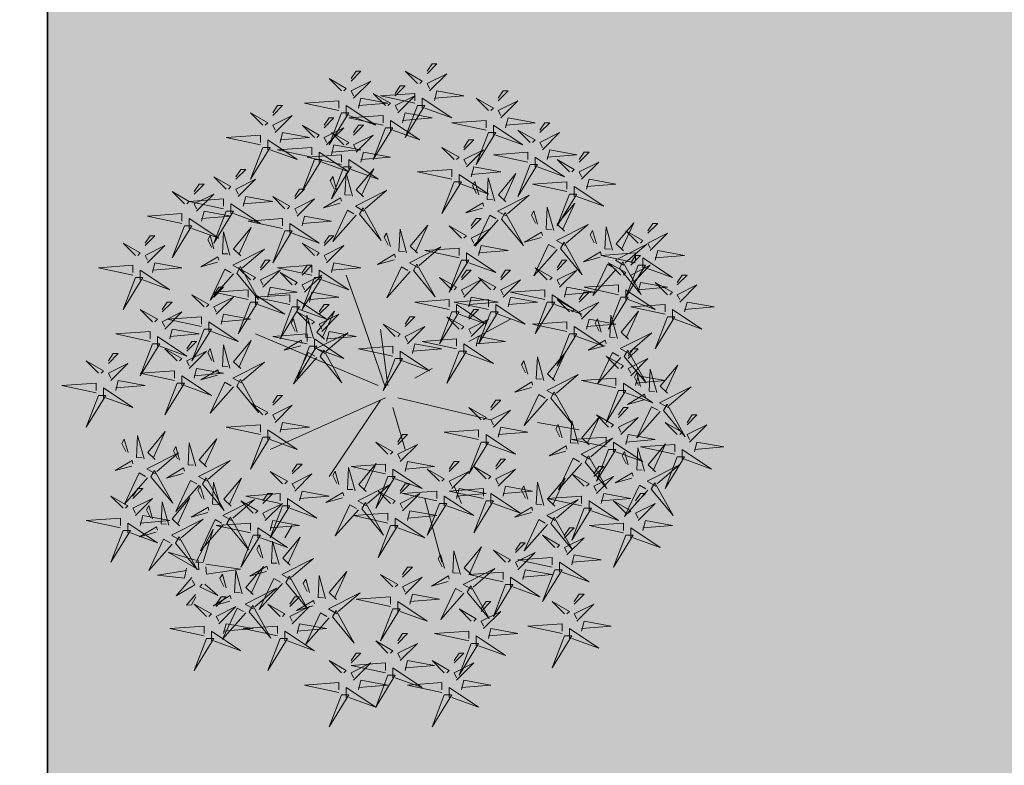
# Model space of a CAD drawing. Units: inches. Extents: x 1704 to 6393, y -157 to 1172.
# Tile 64 of 122: x 1897 to 1937, y 920 to 950. Entities that reach past the tile are written whole.
import ezdxf

# ---------------------------------------------------------------- set-up
doc = ezdxf.new("R2010")
doc.units = ezdxf.units.IN
doc.header["$MEASUREMENT"] = 0
for name, color, linetype, lineweight in [('A-ANNO-DIMS', 7, 'Continuous', 13), ('C-PROP', 7, 'Continuous', 35), ('L-shrub', 74, 'Continuous', 18)]:
    doc.layers.add(name, color=color, linetype=linetype, lineweight=lineweight)
doc.layers.add('L-HRDS-PATT', color=9, linetype='Continuous', lineweight=13, true_color=0xc5c1ba)
doc.styles.get("Standard").update_dxf_attribs({"font": 'arial.ttf'})
doc.dimstyles.get("Standard").update_dxf_attribs({"dimtxt": 6, "dimasz": 2, "dimexe": 0.18, "dimexo": 0.0625, "dimgap": 0.09, "dimtad": 0, "dimtih": 1, "dimtoh": 1, "dimdec": 1, "dimzin": 0, "dimdsep": 46, "dimlunit": 3, "dimtxsty": 'Standard', "dimblk": 'ARCHTICK', "dimcen": 0.09, "dimadec": 0, "dimazin": 0, "dimtfac": 1, "dimtdec": 1, "dimtofl": 0, "dimtmove": 0, "dimatfit": 3, "dimfxl": 1, "dimtolj": 1, "dimtzin": 0, "dimarcsym": 0})

# ---------------------------------------------------------------- blocks, each defined once
blk = doc.blocks.new('autumn shrub')
at = {"layer": 'L-shrub'}
for p, q in [((11.54, 1.92), (51.94, 98)), ((1.92, -3.84), (-38.48, 86.47)), ((-98.12, 69.17), (-107.74, 74.94)), ((0, 0), (-59.64, 40.35)), ((71.18, 17.29), (98.12, 26.9)), ((9.62, -3.84), (71.18, 17.29)), ((11.54, -5.76), (55.79, 0)), ((-5.77, -9.61), (-38.48, -19.21)), ((1.92, -13.45), (-15.39, -86.47)), ((17.31, -26.9), (25.01, -40.35)), ((-76.95, -34.59), (-126.97, -48.04)), ((-67.33, -57.64), (-80.8, -63.41)), ((46.17, -69.17), (63.49, -101.84)), ((-17.31, -122.97), (-23.09, -155.64))]:
    blk.add_line(p, q, dxfattribs=at)
for points in [[(5.77, 222.89), (11.54, 249.79), (13.47, 222.89), (7.7, 222.89)], [(-100.04, 203.68), (-94.27, 230.58), (-92.34, 203.68), (-98.12, 203.68)], [(3.85, 220.97), (-21.16, 230.58), (3.85, 215.21), (3.85, 220.97)], [(21.16, 220.97), (30.78, 230.58), (23.09, 217.13), (21.16, 219.05)], [(1.92, 217.13), (9.62, 217.13), (-5.77, 194.07), (1.92, 215.21)], [(98.12, 194.07), (103.89, 220.97), (105.81, 194.07), (100.04, 194.07)], [(-101.96, 201.75), (-126.97, 211.36), (-101.96, 195.99), (-101.96, 201.75)], [(-84.65, 201.75), (-75.03, 211.36), (-82.73, 197.91), (-84.65, 199.83)], [(15.39, 211.36), (28.86, 197.91), (21.16, 213.28), (17.31, 211.36)], [(28.86, 213.28), (36.55, 205.6), (36.55, 209.44), (30.78, 213.28)], [(-60.75, 182.51), (-81.34, 200.76), (-56.96, 189.22), (-59.8, 184.19)], [(-51.51, 194.97), (-55.15, 208.07), (-47.22, 194.76), (-49.84, 194.03)], [(-41.04, 197.9), (-30.56, 200.83), (-33.91, 202.71), (-40.09, 199.58)], [(7.7, 207.52), (15.39, 205.6), (11.54, 184.46), (9.62, 207.52)], [(46.17, 180.62), (51.94, 207.52), (53.87, 180.62), (48.1, 180.62)], [(96.19, 192.15), (71.18, 201.75), (96.19, 186.38), (96.19, 192.15)], [(113.51, 192.15), (123.13, 201.75), (115.43, 188.3), (113.51, 190.23)], [(-103.89, 197.91), (-96.19, 197.91), (-111.58, 174.85), (-103.89, 195.99)], [(-90.42, 192.15), (-76.95, 178.7), (-84.65, 194.07), (-88.5, 192.15)], [(-76.95, 194.07), (-69.26, 186.38), (-69.26, 190.23), (-75.03, 194.07)], [(-103.45, 175.76), (-107.1, 188.86), (-99.16, 175.55), (-101.78, 174.81)], [(-98.12, 188.3), (-90.42, 186.38), (-94.27, 165.25), (-96.19, 188.3)], [(-45.98, 185.23), (-27.65, 190.35), (-44.82, 191.2), (-45.03, 186.9)], [(15.39, 161.4), (21.16, 188.3), (23.09, 161.4), (17.31, 161.4)], [(44.25, 178.7), (19.24, 188.3), (44.25, 172.93), (44.25, 178.7)], [(61.56, 178.7), (71.18, 188.3), (63.49, 174.85), (61.56, 176.78)], [(94.27, 188.3), (101.96, 188.3), (86.57, 165.25), (94.27, 186.38)], [(-112.69, 163.3), (-133.28, 181.54), (-108.91, 170), (-111.74, 164.97)], [(-92.98, 178.69), (-82.5, 181.61), (-85.85, 183.5), (-92.03, 180.36)], [(-60.02, 179.89), (-80.67, 162.83), (-55, 177.06), (-60.02, 179.89)], [(-57.62, 176.33), (-53.83, 183.03), (-41.31, 158.3), (-55.94, 175.38)], [(-46.41, 176.64), (-40.96, 182.39), (-24.44, 168.66), (-45.47, 178.31)], [(100.04, 178.7), (107.74, 176.78), (103.89, 155.64), (101.96, 178.7)], [(107.74, 182.54), (121.2, 169.09), (113.51, 184.46), (109.66, 182.54)], [(121.2, 184.46), (128.9, 176.78), (128.9, 180.62), (123.13, 184.46)], [(138.52, 155.64), (144.29, 182.54), (146.21, 155.64), (140.44, 155.64)], [(-131.51, 152.18), (-139.33, 153.55), (-136.98, 174.91), (-133.43, 152.04)], [(-97.92, 166.01), (-79.59, 171.13), (-96.76, 171.98), (-96.98, 167.69)], [(42.32, 174.85), (50.02, 174.85), (34.63, 151.8), (42.32, 172.93)], [(55.79, 169.09), (69.26, 155.64), (61.56, 171.01), (57.72, 169.09)], [(69.26, 171.01), (76.95, 163.33), (76.95, 167.17), (71.18, 171.01)], [(-184.69, 138.35), (-178.92, 165.25), (-176.99, 138.35), (-182.77, 138.35)], [(-125.08, 143), (-132.76, 142.46), (-119.03, 166.55), (-125.21, 144.92)], [(-109.56, 157.11), (-105.78, 163.82), (-93.26, 139.08), (-107.89, 156.17)], [(-98.36, 157.42), (-92.9, 163.18), (-76.38, 149.44), (-97.41, 159.1)], [(-57.28, 154.62), (-60.92, 167.72), (-52.99, 154.41), (-55.61, 153.68)], [(-46.81, 157.55), (-36.33, 160.48), (-39.68, 162.36), (-45.86, 159.22)], [(13.47, 159.48), (-11.54, 169.09), (13.47, 153.72), (13.47, 159.48)], [(30.78, 159.48), (40.4, 169.09), (32.71, 155.64), (30.78, 157.56)], [(48.1, 165.25), (55.79, 163.33), (51.94, 142.19), (50.02, 165.25)], [(57.72, 140.27), (63.49, 167.17), (65.41, 140.27), (59.64, 140.27)], [(136.59, 153.72), (111.58, 163.33), (136.59, 147.95), (136.59, 153.72)], [(153.91, 153.72), (163.53, 163.33), (155.83, 149.87), (153.91, 151.8)], [(-138.92, 147.8), (-153.3, 160.27), (-144.54, 145.48), (-140.84, 147.67)], [(-111.96, 160.68), (-132.62, 143.61), (-106.94, 157.85), (-111.96, 160.68)], [(-66.52, 142.16), (-87.11, 160.4), (-62.74, 148.86), (-65.57, 143.84)], [(11.54, 155.64), (19.24, 155.64), (3.85, 132.58), (11.54, 153.72)], [(-152.22, 144.94), (-160.44, 152.06), (-160.16, 148.23), (-154.14, 144.8)], [(-88.06, 135.41), (-91.71, 148.51), (-83.77, 135.2), (-86.39, 134.46)], [(-51.75, 144.88), (-33.42, 150), (-50.59, 150.85), (-50.8, 146.55)], [(25.01, 149.87), (38.48, 136.42), (30.78, 151.8), (26.93, 149.87)], [(55.79, 138.35), (30.78, 147.95), (55.79, 132.58), (55.79, 138.35)], [(38.48, 151.8), (46.17, 144.11), (46.17, 147.95), (40.4, 151.8)], [(73.11, 138.35), (82.73, 147.95), (75.03, 134.5), (73.11, 136.42)], [(134.67, 149.87), (142.36, 149.87), (126.97, 126.82), (134.67, 147.95)], [(150.06, 122.97), (155.83, 149.87), (157.76, 122.97), (151.98, 122.97)], [(-186.61, 136.42), (-211.62, 146.03), (-186.61, 130.66), (-186.61, 136.42)], [(-169.3, 136.42), (-159.68, 146.03), (-167.38, 132.58), (-169.3, 134.5)], [(-144, 137.81), (-152.92, 127.55), (-146.19, 141.51), (-144.13, 139.73)], [(-126.73, 139.03), (-101.1, 131.22), (-127.13, 144.78), (-126.73, 139.03)], [(-97.3, 122.95), (-117.89, 141.19), (-93.52, 129.65), (-96.35, 124.62)], [(-65.79, 139.54), (-86.44, 122.48), (-60.77, 136.71), (-65.79, 139.54)], [(-77.59, 138.33), (-67.11, 141.26), (-70.46, 143.15), (-76.64, 140.01)], [(-63.39, 135.98), (-59.61, 142.68), (-47.08, 117.95), (-61.71, 135.03)], [(-52.18, 136.28), (-46.73, 142.04), (-30.21, 128.31), (-51.24, 137.96)], [(19.67, 127.72), (16.03, 140.82), (23.96, 127.51), (21.35, 126.78)], [(17.31, 146.03), (25.01, 144.11), (21.16, 122.97), (19.24, 146.03)], [(108.17, 127.72), (104.53, 140.82), (112.46, 127.51), (109.84, 126.78)], [(140.44, 140.27), (148.14, 138.35), (144.29, 117.21), (142.36, 140.27)], [(148.14, 144.11), (161.6, 130.66), (153.91, 146.03), (150.06, 144.11)], [(161.6, 146.03), (169.3, 138.35), (169.3, 142.19), (163.53, 146.03)], [(-188.54, 132.58), (-180.84, 132.58), (-196.23, 109.52), (-188.54, 130.66)], [(-157.32, 118.11), (-160.96, 131.21), (-153.03, 117.9), (-155.65, 117.17)], [(-128.51, 136.98), (-132.37, 109.74), (-136.19, 136.44), (-130.43, 136.85)], [(-82.53, 125.66), (-64.2, 130.78), (-81.37, 131.63), (-81.59, 127.34)], [(10.44, 115.26), (-10.16, 133.5), (14.22, 121.96), (11.38, 116.94)], [(30.15, 130.65), (40.62, 133.58), (37.28, 135.46), (31.09, 132.32)], [(53.87, 134.5), (61.56, 134.5), (46.17, 111.45), (53.87, 132.58)], [(98.93, 115.26), (78.34, 133.5), (102.71, 121.96), (99.88, 116.94)], [(118.64, 130.65), (129.12, 133.58), (125.77, 135.46), (119.59, 132.32)], [(-166.56, 105.65), (-187.15, 123.9), (-162.78, 112.36), (-165.61, 107.33)], [(-175.07, 126.82), (-161.6, 113.37), (-169.3, 128.74), (-173.15, 126.82)], [(-161.6, 128.74), (-153.91, 121.05), (-153.91, 124.9), (-159.68, 128.74)], [(-146.85, 121.04), (-136.37, 123.97), (-139.72, 125.86), (-145.9, 122.72)], [(-103.89, 101.84), (-98.12, 128.74), (-96.19, 101.84), (-101.96, 101.84)], [(-94.17, 116.76), (-90.39, 123.47), (-77.87, 98.73), (-92.49, 115.82)], [(25.2, 117.98), (43.54, 123.1), (26.37, 123.95), (26.15, 119.65)], [(59.64, 124.9), (67.33, 122.97), (63.49, 101.84), (61.56, 124.9)], [(67.33, 128.74), (80.8, 115.29), (73.11, 130.66), (69.26, 128.74)], [(78.88, 103.76), (84.65, 130.66), (86.57, 103.76), (80.8, 103.76)], [(80.8, 130.66), (88.5, 122.97), (88.5, 126.82), (82.73, 130.66)], [(113.7, 117.98), (132.03, 123.1), (114.86, 123.95), (114.65, 119.65)], [(148.14, 121.05), (123.13, 130.66), (148.14, 115.29), (148.14, 121.05)], [(165.45, 121.05), (175.07, 130.66), (167.38, 117.21), (165.45, 119.13)], [(-182.77, 122.97), (-175.07, 121.05), (-178.92, 99.92), (-180.84, 122.97)], [(-96.57, 120.33), (-117.23, 103.26), (-91.55, 117.49), (-96.57, 120.33)], [(-82.96, 117.07), (-77.51, 122.83), (-60.99, 109.09), (-82.02, 118.75)], [(-26.93, 94.15), (-21.16, 121.05), (-19.24, 94.15), (-25.01, 94.15)], [(13.57, 109.08), (17.35, 115.78), (29.87, 91.05), (15.24, 108.13)], [(102.06, 109.08), (105.85, 115.78), (118.37, 91.05), (103.74, 108.13)], [(146.21, 117.21), (153.91, 117.21), (138.52, 94.15), (146.21, 115.29)], [(200.08, 94.15), (205.85, 121.05), (207.78, 94.15), (202, 94.15)], [(-151.79, 108.37), (-133.46, 113.49), (-150.63, 114.34), (-150.84, 110.04)], [(-105.81, 99.92), (-130.82, 109.52), (-105.81, 94.15), (-105.81, 99.92)], [(-88.5, 99.92), (-78.88, 109.52), (-86.57, 96.07), (-88.5, 98)], [(11.17, 112.64), (-9.49, 95.58), (16.19, 109.81), (11.17, 112.64)], [(24.77, 109.38), (30.23, 115.14), (46.74, 101.41), (25.72, 111.06)], [(76.95, 101.84), (51.94, 111.45), (76.95, 96.07), (76.95, 101.84)], [(99.66, 112.64), (79.01, 95.58), (104.68, 109.81), (99.66, 112.64)], [(94.27, 101.84), (103.89, 111.45), (96.19, 98), (94.27, 99.92)], [(113.27, 109.38), (118.72, 115.14), (135.24, 101.41), (114.21, 111.06)], [(159.68, 111.45), (173.15, 98), (165.45, 113.37), (161.6, 111.45)], [(173.15, 113.37), (180.84, 105.68), (180.84, 109.52), (175.07, 113.37)], [(-165.83, 103.03), (-186.48, 85.97), (-160.81, 100.2), (-165.83, 103.03)], [(-184.69, 80.7), (-178.92, 107.6), (-176.99, 80.7), (-182.77, 80.7)], [(-163.43, 99.47), (-159.65, 106.17), (-147.12, 81.44), (-161.75, 98.53)], [(-152.22, 99.78), (-146.77, 105.54), (-130.25, 91.8), (-151.28, 101.45)], [(-134.24, 89.29), (-137.88, 102.39), (-129.94, 89.08), (-132.56, 88.35)], [(-80.8, 78.78), (-75.03, 105.68), (-73.11, 78.78), (-78.88, 78.78)], [(-28.86, 92.23), (-53.87, 101.84), (-28.86, 86.47), (-28.86, 92.23)], [(-11.54, 92.23), (-1.92, 101.84), (-9.62, 88.39), (-11.54, 90.31)], [(134.67, 76.86), (140.44, 103.76), (142.36, 76.86), (136.59, 76.86)], [(151.98, 107.6), (159.68, 105.68), (155.83, 84.54), (153.91, 107.6)], [(198.16, 92.23), (173.15, 101.84), (198.16, 86.47), (198.16, 92.23)], [(215.47, 92.23), (225.09, 101.84), (217.4, 88.39), (215.47, 90.31)], [(-143.47, 76.83), (-164.07, 95.07), (-139.69, 83.53), (-142.53, 78.51)], [(-123.76, 92.22), (-113.29, 95.15), (-116.63, 97.03), (-122.82, 93.89)], [(-107.74, 96.07), (-100.04, 96.07), (-115.43, 73.02), (-107.74, 94.15)], [(75.03, 98), (82.73, 98), (67.33, 74.94), (75.03, 96.07)], [(75.03, 71.09), (80.8, 98), (82.73, 71.09), (76.95, 71.09)], [(88.5, 92.23), (101.96, 78.78), (94.27, 94.15), (90.42, 92.23)], [(101.96, 94.15), (109.66, 86.47), (109.66, 90.31), (103.89, 94.15)], [(-186.61, 78.78), (-211.62, 88.39), (-186.61, 73.02), (-186.61, 78.78)], [(-169.3, 78.78), (-159.68, 88.39), (-167.38, 74.94), (-169.3, 76.86)], [(-128.7, 79.55), (-110.37, 84.67), (-127.54, 85.52), (-127.76, 81.22)], [(-82.73, 76.86), (-107.74, 86.47), (-82.73, 71.09), (-82.73, 76.86)], [(-101.96, 86.47), (-94.27, 84.54), (-98.12, 63.41), (-100.04, 86.47)], [(-94.27, 90.31), (-80.8, 76.86), (-88.5, 92.23), (-92.34, 90.31)], [(-80.8, 92.23), (-73.11, 84.54), (-73.11, 88.39), (-78.88, 92.23)], [(-65.41, 76.86), (-55.79, 86.47), (-63.49, 73.02), (-65.41, 74.94)], [(-30.78, 88.39), (-23.09, 88.39), (-38.48, 65.33), (-30.78, 86.47)], [(80.8, 88.39), (88.5, 86.47), (84.65, 65.33), (82.73, 88.39)], [(196.23, 88.39), (203.93, 88.39), (188.54, 65.33), (196.23, 86.47)], [(-140.34, 70.65), (-136.56, 77.35), (-124.04, 52.62), (-138.67, 69.7)], [(-25.01, 78.78), (-17.31, 76.86), (-21.16, 55.72), (-23.09, 78.78)], [(-17.31, 82.62), (-3.85, 69.17), (-11.54, 84.54), (-15.39, 82.62)], [(-3.85, 84.54), (3.85, 76.86), (3.85, 80.7), (-1.92, 84.54)], [(44.25, 57.64), (50.02, 84.54), (51.94, 57.64), (46.17, 57.64)], [(73.11, 69.17), (48.1, 78.78), (73.11, 63.41), (73.11, 69.17)], [(90.42, 69.17), (100.04, 78.78), (92.34, 65.33), (90.42, 67.25)], [(98.12, 53.8), (103.89, 80.7), (105.81, 53.8), (100.04, 53.8)], [(132.75, 74.94), (107.74, 84.54), (132.75, 69.17), (132.75, 74.94)], [(150.06, 74.94), (159.68, 84.54), (151.98, 71.09), (150.06, 73.02)], [(190.46, 53.8), (196.23, 80.7), (198.16, 53.8), (192.39, 53.8)], [(202, 78.78), (209.7, 76.86), (205.85, 55.72), (203.93, 78.78)], [(209.7, 82.62), (223.17, 69.17), (215.47, 84.54), (211.62, 82.62)], [(223.17, 84.54), (230.86, 76.86), (230.86, 80.7), (225.09, 84.54)], [(-188.54, 74.94), (-180.84, 74.94), (-196.23, 51.88), (-188.54, 73.02)], [(-175.07, 69.17), (-161.6, 55.72), (-169.3, 71.09), (-173.15, 69.17)], [(-142.74, 74.21), (-163.4, 57.15), (-137.72, 71.38), (-142.74, 74.21)], [(-161.6, 71.09), (-153.91, 63.41), (-153.91, 67.25), (-159.68, 71.09)], [(-129.14, 70.95), (-123.68, 76.71), (-107.16, 62.98), (-128.19, 72.63)], [(-84.65, 73.02), (-76.95, 73.02), (-92.34, 49.96), (-84.65, 71.09)], [(42.76, 62.39), (39.12, 75.49), (47.05, 62.18), (44.43, 61.45)], [(53.23, 65.32), (63.71, 68.25), (60.36, 70.13), (54.18, 66.99)], [(130.82, 71.09), (138.52, 71.09), (123.13, 48.04), (130.82, 69.17)], [(-182.77, 65.33), (-175.07, 63.41), (-178.92, 42.27), (-180.84, 65.33)], [(-161.17, 52.78), (-164.81, 65.88), (-156.88, 52.57), (-159.5, 51.84)], [(-78.88, 63.41), (-71.18, 61.49), (-75.03, 40.35), (-76.95, 63.41)], [(-71.18, 67.25), (-57.72, 53.8), (-65.41, 69.17), (-69.26, 67.25)], [(-57.72, 69.17), (-50.02, 61.49), (-50.02, 65.33), (-55.79, 69.17)], [(33.52, 49.93), (12.93, 68.17), (37.3, 56.63), (34.47, 51.61)], [(42.32, 55.72), (17.31, 65.33), (42.32, 49.96), (42.32, 55.72)], [(59.64, 55.72), (69.26, 65.33), (61.56, 51.88), (59.64, 53.8)], [(71.18, 65.33), (78.88, 65.33), (63.49, 42.27), (71.18, 63.41)], [(144.29, 65.33), (157.76, 51.88), (150.06, 67.25), (146.21, 65.33)], [(157.76, 67.25), (165.45, 59.57), (165.45, 63.41), (159.68, 67.25)], [(-228.94, 32.67), (-223.17, 59.57), (-221.24, 32.67), (-227.01, 32.67)], [(-170.4, 40.32), (-191, 58.57), (-166.62, 47.03), (-169.46, 42)], [(-150.69, 55.71), (-140.22, 58.64), (-143.57, 60.53), (-149.75, 57.39)], [(48.29, 52.64), (66.62, 57.77), (49.45, 58.62), (49.24, 54.32)], [(96.19, 51.88), (71.18, 61.49), (96.19, 46.12), (96.19, 51.88)], [(76.95, 55.72), (84.65, 53.8), (80.8, 32.67), (78.88, 55.72)], [(84.65, 59.57), (98.12, 46.12), (90.42, 61.49), (86.57, 59.57)], [(98.12, 61.49), (105.81, 53.8), (105.81, 57.64), (100.04, 61.49)], [(113.51, 51.88), (123.13, 61.49), (115.43, 48.04), (113.51, 49.96)], [(136.59, 61.49), (144.29, 59.57), (140.44, 38.43), (138.52, 61.49)], [(188.54, 51.88), (163.53, 61.49), (188.54, 46.12), (188.54, 51.88)], [(184.69, 30.74), (190.46, 57.64), (192.39, 30.74), (186.61, 30.74)], [(205.85, 51.88), (215.47, 61.49), (207.78, 48.04), (205.85, 49.96)], [(227.01, 32.67), (232.79, 59.57), (234.71, 32.67), (228.94, 32.67)], [(-155.64, 43.04), (-137.31, 48.16), (-154.48, 49.01), (-154.69, 44.71)], [(34.25, 47.31), (13.6, 30.25), (39.27, 44.48), (34.25, 47.31)], [(40.4, 51.88), (48.1, 51.88), (32.71, 28.82), (40.4, 49.96)], [(36.65, 43.75), (40.43, 50.45), (52.96, 25.72), (38.33, 42.8)], [(47.86, 44.05), (53.31, 49.81), (69.83, 36.08), (48.8, 45.73)], [(53.87, 46.12), (67.33, 32.67), (59.64, 48.04), (55.79, 46.12)], [(67.33, 48.04), (75.03, 40.35), (75.03, 44.19), (69.26, 48.04)], [(94.27, 48.04), (101.96, 48.04), (86.57, 24.98), (94.27, 46.12)], [(186.61, 48.04), (194.31, 48.04), (178.92, 24.98), (186.61, 46.12)], [(-230.86, 30.74), (-255.87, 40.35), (-230.86, 24.98), (-230.86, 30.74)], [(-213.55, 30.74), (-203.93, 40.35), (-211.62, 26.9), (-213.55, 28.82)], [(-167.27, 34.14), (-163.49, 40.84), (-150.97, 16.11), (-165.6, 33.2)], [(-156.07, 34.45), (-150.62, 40.21), (-134.1, 26.47), (-155.13, 36.12)], [(-76.52, 29.73), (-80.16, 42.83), (-72.23, 29.51), (-74.85, 28.78)], [(46.17, 42.27), (53.87, 40.35), (50.02, 19.21), (48.1, 42.27)], [(107.74, 42.27), (121.2, 28.82), (113.51, 44.19), (109.66, 42.27)], [(121.2, 44.19), (128.9, 36.51), (128.9, 40.35), (123.13, 44.19)], [(154.34, 31.65), (150.7, 44.75), (158.63, 31.44), (156.02, 30.7)], [(164.82, 34.57), (175.29, 37.5), (171.94, 39.39), (165.76, 36.25)], [(200.08, 42.27), (213.55, 28.82), (205.85, 44.19), (202, 42.27)], [(225.09, 30.74), (200.08, 40.35), (225.09, 24.98), (225.09, 30.74)], [(213.55, 44.19), (221.24, 36.51), (221.24, 40.35), (215.47, 44.19)], [(242.41, 30.74), (252.02, 40.35), (244.33, 26.9), (242.41, 28.82)], [(-169.68, 37.7), (-190.33, 20.64), (-164.66, 34.87), (-169.68, 37.7)], [(-85.76, 17.27), (-106.35, 35.51), (-81.97, 23.97), (-84.81, 18.94)], [(-66.05, 32.65), (-55.57, 35.58), (-58.92, 37.47), (-65.1, 34.33)], [(100.04, 38.43), (107.74, 36.51), (103.89, 15.37), (101.96, 38.43)], [(145.11, 19.19), (124.51, 37.43), (148.89, 25.89), (146.05, 20.86)], [(182.77, 28.82), (157.76, 38.43), (182.77, 23.06), (182.77, 28.82)], [(192.39, 38.43), (200.08, 36.51), (196.23, 15.37), (194.31, 38.43)], [(200.08, 28.82), (209.7, 38.43), (202, 24.98), (200.08, 26.9)], [(-232.79, 26.9), (-225.09, 26.9), (-240.48, 3.84), (-232.79, 24.98)], [(-70.99, 19.98), (-52.66, 25.1), (-69.83, 25.95), (-70.04, 21.66)], [(159.87, 21.9), (178.21, 27.02), (161.04, 27.87), (160.82, 23.58)], [(180.84, 24.98), (188.54, 24.98), (173.15, 1.92), (180.84, 23.06)], [(223.17, 26.9), (230.86, 26.9), (215.47, 3.84), (223.17, 24.98)], [(215.47, -1.92), (221.24, 24.98), (223.17, -1.92), (217.4, -1.92)], [(-227.01, 17.29), (-219.32, 15.37), (-223.17, -5.76), (-225.09, 17.29)], [(-219.32, 21.14), (-205.85, 7.69), (-213.55, 23.06), (-217.4, 21.14)], [(-213.55, -3.84), (-207.78, 23.06), (-205.85, -3.84), (-211.62, -3.84)], [(-205.85, 23.06), (-198.16, 15.37), (-198.16, 19.21), (-203.93, 23.06)], [(-161.6, -7.69), (-155.83, 19.21), (-153.91, -7.69), (-159.68, -7.69)], [(-96.19, -5.76), (-90.42, 21.14), (-88.5, -5.76), (-94.27, -5.76)], [(-82.63, 11.08), (-78.84, 17.78), (-66.32, -6.95), (-80.95, 10.14)], [(-71.42, 11.39), (-65.97, 17.15), (-49.45, 3.41), (-70.48, 13.06)], [(-57.72, -3.84), (-51.94, 23.06), (-50.02, -3.84), (-55.79, -3.84)], [(34.63, -9.61), (40.4, 17.29), (42.32, -9.61), (36.55, -9.61)], [(145.83, 16.57), (125.18, -0.5), (150.86, 13.74), (145.83, 16.57)], [(148.24, 13), (152.02, 19.71), (164.54, -5.03), (149.91, 12.06)], [(159.44, 13.31), (164.89, 19.07), (181.41, 5.33), (160.39, 14.99)], [(194.31, 19.21), (207.78, 5.76), (200.08, 21.14), (196.23, 19.21)], [(207.78, 21.14), (215.47, 13.45), (215.47, 17.29), (209.7, 21.14)], [(228.94, 17.29), (236.63, 15.37), (232.79, -5.76), (230.86, 17.29)], [(236.63, 21.14), (250.1, 7.69), (242.41, 23.06), (238.56, 21.14)], [(250.1, 23.06), (257.8, 15.37), (257.8, 19.21), (252.02, 23.06)], [(-85.03, 14.65), (-105.68, -2.42), (-80.01, 11.81), (-85.03, 14.65)], [(186.61, 15.37), (194.31, 13.45), (190.46, -7.69), (188.54, 15.37)], [(-215.47, -5.76), (-240.48, 3.84), (-215.47, -11.53), (-215.47, -5.76)], [(-198.16, -5.76), (-188.54, 3.84), (-196.23, -9.61), (-198.16, -7.69)], [(-163.53, -9.61), (-188.54, 0), (-163.53, -15.37), (-163.53, -9.61)], [(-146.21, -9.61), (-136.59, 0), (-144.29, -13.45), (-146.21, -11.53)], [(-98.12, -7.69), (-123.13, 1.92), (-98.12, -13.45), (-98.12, -7.69)], [(-59.64, -5.76), (-84.65, 3.84), (-59.64, -11.53), (-59.64, -5.76)], [(-80.8, -7.69), (-71.18, 1.92), (-78.88, -11.53), (-80.8, -9.61)], [(-42.32, -5.76), (-32.71, 3.84), (-40.4, -9.61), (-42.32, -7.69)], [(110.09, -10.62), (106.45, 2.47), (114.39, -10.84), (111.77, -11.57)], [(213.55, -3.84), (188.54, 5.76), (213.55, -9.61), (213.55, -3.84)], [(230.86, -3.84), (240.48, 5.76), (232.79, -7.69), (230.86, -5.76)], [(232.79, -26.9), (238.56, 0), (240.48, -26.9), (234.71, -26.9)], [(32.71, -11.53), (7.7, -1.92), (32.71, -17.29), (32.71, -11.53)], [(50.02, -11.53), (59.64, -1.92), (51.94, -15.37), (50.02, -13.45)], [(100.86, -23.09), (80.26, -4.84), (104.64, -16.38), (101.8, -21.41)], [(120.57, -7.7), (131.04, -4.77), (127.7, -2.88), (121.51, -6.02)], [(211.62, -7.69), (219.32, -7.69), (203.93, -30.74), (211.62, -9.61)], [(-217.4, -9.61), (-209.7, -9.61), (-225.09, -32.67), (-217.4, -11.53)], [(-203.93, -15.37), (-190.46, -28.82), (-198.16, -13.45), (-202, -15.37)], [(-190.46, -13.45), (-182.77, -21.14), (-182.77, -17.29), (-188.54, -13.45)], [(-165.45, -13.45), (-157.76, -13.45), (-173.15, -36.51), (-165.45, -15.37)], [(-100.04, -11.53), (-92.34, -11.53), (-107.74, -34.59), (-100.04, -13.45)], [(-86.57, -17.29), (-73.11, -30.74), (-80.8, -15.37), (-84.65, -17.29)], [(-73.11, -15.37), (-65.41, -23.06), (-65.41, -19.21), (-71.18, -15.37)], [(-61.56, -9.61), (-53.87, -9.61), (-69.26, -32.67), (-61.56, -11.53)], [(-48.1, -15.37), (-34.63, -28.82), (-42.32, -13.45), (-46.17, -15.37)], [(-34.63, -13.45), (-26.93, -21.14), (-26.93, -17.29), (-32.71, -13.45)], [(30.78, -15.37), (38.48, -15.37), (23.09, -38.43), (30.78, -17.29)], [(115.63, -20.37), (133.96, -15.25), (116.79, -14.4), (116.57, -18.7)], [(225.09, -13.45), (238.56, -26.9), (230.86, -11.53), (227.01, -13.45)], [(238.56, -11.53), (246.25, -19.21), (246.25, -15.37), (240.48, -11.53)], [(-228.94, -48.04), (-223.17, -21.14), (-221.24, -48.04), (-227.01, -48.04)], [(-211.62, -19.21), (-203.93, -21.14), (-207.78, -42.27), (-209.7, -19.21)], [(-159.68, -23.06), (-151.98, -24.98), (-155.83, -46.12), (-157.76, -23.06)], [(-151.98, -19.21), (-138.52, -32.67), (-146.21, -17.29), (-150.06, -19.21)], [(-138.52, -17.29), (-130.82, -24.98), (-130.82, -21.14), (-136.59, -17.29)], [(-94.27, -21.14), (-86.57, -23.06), (-90.42, -44.19), (-92.34, -21.14)], [(-78.88, -44.19), (-73.11, -17.29), (-71.18, -44.19), (-76.95, -44.19)], [(-55.79, -19.21), (-48.1, -21.14), (-51.94, -42.27), (-53.87, -19.21)], [(44.25, -21.14), (57.72, -34.59), (50.02, -19.21), (46.17, -21.14)], [(57.72, -19.21), (65.41, -26.9), (65.41, -23.06), (59.64, -19.21)], [(103.99, -29.27), (107.77, -22.57), (120.29, -47.3), (105.66, -30.21)], [(230.86, -28.82), (205.85, -19.21), (230.86, -34.59), (230.86, -28.82)], [(217.4, -17.29), (225.09, -19.21), (221.24, -40.35), (219.32, -17.29)], [(248.18, -28.82), (257.8, -19.21), (250.1, -32.67), (248.18, -30.74)], [(36.55, -24.98), (44.25, -26.9), (40.4, -48.04), (38.48, -24.98)], [(71.18, -53.8), (76.95, -26.9), (78.88, -53.8), (73.11, -53.8)], [(101.59, -25.71), (80.93, -42.77), (106.61, -28.54), (101.59, -25.71)], [(115.19, -28.96), (120.65, -23.2), (137.17, -36.94), (116.14, -27.29)], [(173.15, -55.72), (178.92, -28.82), (180.84, -55.72), (175.07, -55.72)], [(-80.8, -46.12), (-105.81, -36.51), (-80.8, -51.88), (-80.8, -46.12)], [(-63.49, -46.12), (-53.87, -36.51), (-61.56, -49.96), (-63.49, -48.04)], [(40.4, -59.57), (46.17, -32.67), (48.1, -59.57), (42.32, -59.57)], [(111.58, -61.49), (117.35, -34.59), (119.28, -61.49), (113.51, -61.49)], [(228.94, -32.67), (236.63, -32.67), (221.24, -55.72), (228.94, -34.59)], [(242.41, -38.43), (255.87, -51.88), (248.18, -36.51), (244.33, -38.43)], [(255.87, -36.51), (263.57, -44.19), (263.57, -40.35), (257.8, -36.51)], [(-230.86, -49.96), (-255.87, -40.35), (-230.86, -55.72), (-230.86, -49.96)], [(-213.55, -49.96), (-203.93, -40.35), (-211.62, -53.8), (-213.55, -51.88)], [(-188.54, -69.17), (-182.77, -42.27), (-180.84, -69.17), (-186.61, -69.17)], [(-141.93, -52.9), (-145.57, -39.8), (-137.64, -53.11), (-140.26, -53.84)], [(-131.46, -49.97), (-120.98, -47.04), (-124.33, -45.16), (-130.51, -48.29)], [(69.26, -55.72), (44.25, -46.12), (69.26, -61.49), (69.26, -55.72)], [(86.57, -55.72), (96.19, -46.12), (88.5, -59.57), (86.57, -57.64)], [(234.71, -42.27), (242.41, -44.19), (238.56, -65.33), (236.63, -42.27)], [(-232.79, -53.8), (-225.09, -53.8), (-240.48, -76.86), (-232.79, -55.72)], [(-151.17, -65.36), (-171.76, -47.11), (-147.39, -58.66), (-150.22, -63.68)], [(-82.73, -49.96), (-75.03, -49.96), (-90.42, -73.02), (-82.73, -51.88)], [(-76.95, -80.7), (-71.18, -53.8), (-69.26, -80.7), (-75.03, -80.7)], [(-69.26, -55.72), (-55.79, -69.17), (-63.49, -53.8), (-67.33, -55.72)], [(-55.79, -53.8), (-48.1, -61.49), (-48.1, -57.64), (-53.87, -53.8)], [(-30.78, -76.86), (-25.01, -49.96), (-23.09, -76.86), (-28.86, -76.86)], [(38.48, -61.49), (13.47, -51.88), (38.48, -67.25), (38.48, -61.49)], [(55.79, -61.49), (65.41, -51.88), (57.72, -65.33), (55.79, -63.41)], [(109.66, -63.41), (84.65, -53.8), (109.66, -69.17), (109.66, -63.41)], [(126.97, -63.41), (136.59, -53.8), (128.9, -67.25), (126.97, -65.33)], [(171.22, -57.64), (146.21, -48.04), (171.22, -63.41), (171.22, -57.64)], [(188.54, -57.64), (198.16, -48.04), (190.46, -61.49), (188.54, -59.57)], [(-219.32, -59.57), (-205.85, -73.02), (-213.55, -57.64), (-217.4, -59.57)], [(-190.46, -71.09), (-215.47, -61.49), (-190.46, -76.86), (-190.46, -71.09)], [(-205.85, -57.64), (-198.16, -65.33), (-198.16, -61.49), (-203.93, -57.64)], [(-173.15, -71.09), (-163.53, -61.49), (-171.22, -74.94), (-173.15, -73.02)], [(-136.4, -62.64), (-118.07, -57.52), (-135.24, -56.67), (-135.45, -60.97)], [(-76.95, -59.57), (-69.26, -61.49), (-73.11, -82.62), (-75.03, -59.57)], [(67.33, -59.57), (75.03, -59.57), (59.64, -82.62), (67.33, -61.49)], [(71.18, -84.54), (76.95, -57.64), (78.88, -84.54), (73.11, -84.54)], [(169.3, -61.49), (176.99, -61.49), (161.6, -84.54), (169.3, -63.41)], [(211.62, -82.62), (217.4, -55.72), (219.32, -82.62), (213.55, -82.62)], [(-227.01, -63.41), (-219.32, -65.33), (-223.17, -86.47), (-225.09, -63.41)], [(-150.44, -67.98), (-171.09, -85.04), (-145.42, -70.81), (-150.44, -67.98)], [(-148.04, -71.54), (-144.26, -64.84), (-131.73, -89.57), (-146.36, -72.49)], [(-142.36, -96.07), (-136.59, -69.17), (-134.67, -96.07), (-140.44, -96.07)], [(-136.83, -71.23), (-131.38, -65.48), (-114.86, -79.21), (-135.89, -69.56)], [(-32.71, -78.78), (-57.72, -69.17), (-32.71, -84.54), (-32.71, -78.78)], [(-15.39, -78.78), (-5.77, -69.17), (-13.47, -82.62), (-15.39, -80.7)], [(36.55, -65.33), (44.25, -65.33), (28.86, -88.39), (36.55, -67.25)], [(50.02, -71.09), (63.49, -84.54), (55.79, -69.17), (51.94, -71.09)], [(63.49, -69.17), (71.18, -76.86), (71.18, -73.02), (65.41, -69.17)], [(73.11, -69.17), (80.8, -71.09), (76.95, -92.23), (75.03, -69.17)], [(80.8, -65.33), (94.27, -78.78), (86.57, -63.41), (82.73, -65.33)], [(94.27, -63.41), (101.96, -71.09), (101.96, -67.25), (96.19, -63.41)], [(107.74, -67.25), (115.43, -67.25), (100.04, -90.31), (107.74, -69.17)], [(150.49, -79.8), (146.85, -66.7), (154.79, -80.01), (152.17, -80.74)], [(182.77, -67.25), (196.23, -80.7), (188.54, -65.33), (184.69, -67.25)], [(196.23, -65.33), (203.93, -73.02), (203.93, -69.17), (198.16, -65.33)], [(-192.39, -74.94), (-184.69, -74.94), (-200.08, -98), (-192.39, -76.86)], [(-78.88, -82.62), (-103.89, -73.02), (-78.88, -88.39), (-78.88, -82.62)], [(-61.56, -82.62), (-51.94, -73.02), (-59.64, -86.47), (-61.56, -84.54)], [(42.32, -74.94), (50.02, -76.86), (46.17, -98), (44.25, -74.94)], [(69.26, -86.47), (44.25, -76.86), (69.26, -92.23), (69.26, -86.47)], [(86.57, -86.47), (96.19, -76.86), (88.5, -90.31), (86.57, -88.39)], [(113.51, -76.86), (121.2, -78.78), (117.35, -99.92), (115.43, -76.86)], [(141.26, -92.26), (120.66, -74.02), (145.04, -85.56), (142.2, -90.58)], [(121.2, -73.02), (134.67, -86.47), (126.97, -71.09), (123.13, -73.02)], [(134.67, -71.09), (142.36, -78.78), (142.36, -74.94), (136.59, -71.09)], [(160.97, -76.87), (171.44, -73.94), (168.1, -72.06), (161.91, -75.19)], [(175.07, -71.09), (182.77, -73.02), (178.92, -94.15), (176.99, -71.09)], [(209.7, -84.54), (184.69, -74.94), (209.7, -90.31), (209.7, -84.54)], [(227.01, -84.54), (236.63, -74.94), (228.94, -88.39), (227.01, -86.47)], [(-186.61, -84.54), (-178.92, -86.47), (-182.77, -107.6), (-184.69, -84.54)], [(-178.92, -80.7), (-165.45, -94.15), (-173.15, -78.78), (-176.99, -80.7)], [(-165.45, -78.78), (-157.76, -86.47), (-157.76, -82.62), (-163.53, -78.78)], [(-34.63, -82.62), (-26.93, -82.62), (-42.32, -105.68), (-34.63, -84.54)], [(156.03, -89.54), (174.36, -84.42), (157.19, -83.57), (156.97, -87.87)], [(-144.29, -98), (-169.3, -88.39), (-144.29, -103.76), (-144.29, -98)], [(-126.97, -98), (-117.35, -88.39), (-125.05, -101.84), (-126.97, -99.92)], [(-80.8, -86.47), (-73.11, -86.47), (-88.5, -109.52), (-80.8, -88.39)], [(-67.33, -92.23), (-53.87, -105.68), (-61.56, -90.31), (-65.41, -92.23)], [(-53.87, -90.31), (-46.17, -98), (-46.17, -94.15), (-51.94, -90.31)], [(-28.86, -92.23), (-21.16, -94.15), (-25.01, -115.29), (-26.93, -92.23)], [(-21.16, -88.39), (-7.7, -101.84), (-15.39, -86.47), (-19.24, -88.39)], [(-7.7, -86.47), (0, -94.15), (0, -90.31), (-5.77, -86.47)], [(67.33, -90.31), (75.03, -90.31), (59.64, -113.37), (67.33, -92.23)], [(144.39, -98.44), (148.17, -91.74), (160.69, -116.47), (146.06, -99.39)], [(155.59, -98.13), (161.05, -92.38), (177.57, -106.11), (156.54, -96.46)], [(186.61, -115.29), (192.39, -88.39), (194.31, -115.29), (188.54, -115.29)], [(207.78, -88.39), (215.47, -88.39), (200.08, -111.45), (207.78, -90.31)], [(221.24, -94.15), (234.71, -107.6), (227.01, -92.23), (223.17, -94.15)], [(234.71, -92.23), (242.41, -99.92), (242.41, -96.07), (236.63, -92.23)], [(-75.03, -96.07), (-67.33, -98), (-71.18, -119.13), (-73.11, -96.07)], [(73.11, -99.92), (80.8, -101.84), (76.95, -122.97), (75.03, -99.92)], [(80.8, -96.07), (94.27, -109.52), (86.57, -94.15), (82.73, -96.07)], [(94.27, -94.15), (101.96, -101.84), (101.96, -98), (96.19, -94.15)], [(141.99, -94.88), (121.33, -111.94), (147.01, -97.71), (141.99, -94.88)], [(213.55, -98), (221.24, -99.92), (217.4, -121.05), (215.47, -98)], [(-146.21, -101.84), (-138.52, -101.84), (-153.91, -124.9), (-146.21, -103.76)], [(-132.75, -107.6), (-119.28, -121.05), (-126.97, -105.68), (-130.82, -107.6)], [(-130.82, -134.5), (-125.05, -107.6), (-123.13, -134.5), (-128.9, -134.5)], [(-119.28, -105.68), (-111.58, -113.37), (-111.58, -109.52), (-117.35, -105.68)], [(-88.06, -118.23), (-91.71, -105.13), (-83.77, -118.44), (-86.39, -119.17)], [(10.05, -118.23), (6.41, -105.13), (14.35, -118.44), (11.73, -119.17)], [(78.88, -128.74), (84.65, -101.84), (86.57, -128.74), (80.8, -128.74)], [(184.69, -117.21), (159.68, -107.6), (184.69, -122.97), (184.69, -117.21)], [(202, -117.21), (211.62, -107.6), (203.93, -121.05), (202, -119.13)], [(-182.77, -142.19), (-176.99, -115.29), (-175.07, -142.19), (-180.84, -142.19)], [(-140.44, -111.45), (-132.75, -113.37), (-136.59, -134.5), (-138.52, -111.45)], [(-97.3, -130.69), (-117.89, -112.44), (-93.52, -123.99), (-96.35, -129.01)], [(-77.59, -115.3), (-67.11, -112.37), (-70.46, -110.49), (-76.64, -113.62)], [(0.82, -130.69), (-19.78, -112.44), (4.6, -123.99), (1.76, -129.01)], [(20.53, -115.3), (31, -112.37), (27.66, -110.49), (21.47, -113.62)], [(127.41, -125.91), (123.77, -112.81), (131.7, -126.12), (129.08, -126.86)], [(-82.53, -127.97), (-64.2, -122.85), (-81.37, -122), (-81.59, -126.3)], [(15.59, -127.97), (33.92, -122.85), (16.75, -122), (16.53, -126.3)], [(76.95, -130.66), (51.94, -121.05), (76.95, -136.42), (76.95, -130.66)], [(53.87, -146.03), (59.64, -119.13), (61.56, -146.03), (55.79, -146.03)], [(94.27, -130.66), (103.89, -121.05), (96.19, -134.5), (94.27, -132.58)], [(118.17, -138.37), (97.58, -120.13), (121.95, -131.67), (119.12, -136.7)], [(137.88, -122.99), (148.36, -120.06), (145.01, -118.17), (138.83, -121.31)], [(163.53, -146.03), (169.3, -119.13), (171.22, -146.03), (165.45, -146.03)], [(182.77, -121.05), (190.46, -121.05), (175.07, -144.11), (182.77, -122.97)], [(-132.75, -136.42), (-157.76, -126.82), (-132.75, -142.19), (-132.75, -136.42)], [(-115.43, -136.42), (-105.81, -126.82), (-113.51, -140.27), (-115.43, -138.35)], [(-94.17, -136.87), (-90.39, -130.17), (-77.87, -154.9), (-92.49, -137.82)], [(-82.96, -136.56), (-77.51, -130.81), (-60.99, -144.54), (-82.02, -134.89)], [(-82.73, -157.56), (-76.95, -130.66), (-75.03, -157.56), (-80.8, -157.56)], [(3.95, -136.87), (7.73, -130.17), (20.25, -154.9), (5.62, -137.82)], [(15.15, -136.56), (20.61, -130.81), (37.13, -144.54), (16.1, -134.89)], [(132.94, -135.66), (151.27, -130.54), (134.1, -129.69), (133.89, -133.98)], [(188.54, -130.66), (196.23, -132.58), (192.39, -153.72), (190.46, -130.66)], [(196.23, -126.82), (209.7, -140.27), (202, -124.9), (198.16, -126.82)], [(209.7, -124.9), (217.4, -132.58), (217.4, -128.74), (211.62, -124.9)], [(-184.69, -144.11), (-209.7, -134.5), (-184.69, -149.87), (-184.69, -144.11)], [(-167.38, -144.11), (-157.76, -134.5), (-165.45, -147.95), (-167.38, -146.03)], [(-96.57, -133.31), (-117.23, -150.37), (-91.55, -136.14), (-96.57, -133.31)], [(-39.97, -145.13), (-43.61, -132.03), (-35.67, -145.34), (-38.29, -146.07)], [(-29.49, -142.2), (-19.02, -139.27), (-22.36, -137.39), (-28.55, -140.52)], [(1.55, -133.31), (-19.11, -150.37), (6.57, -136.14), (1.55, -133.31)], [(51.94, -147.95), (26.93, -138.35), (51.94, -153.72), (51.94, -147.95)], [(75.03, -134.5), (82.73, -134.5), (67.33, -157.56), (75.03, -136.42)], [(69.26, -147.95), (78.88, -138.35), (71.18, -151.8), (69.26, -149.87)], [(88.5, -140.27), (101.96, -153.72), (94.27, -138.35), (90.42, -140.27)], [(101.96, -138.35), (109.66, -146.03), (109.66, -142.19), (103.89, -138.35)], [(121.3, -144.56), (125.08, -137.85), (137.61, -162.59), (122.98, -145.5)], [(132.51, -144.25), (137.96, -138.49), (154.48, -152.23), (133.45, -142.57)], [(161.6, -147.95), (136.59, -138.35), (161.6, -153.72), (161.6, -147.95)], [(178.92, -147.95), (188.54, -138.35), (180.84, -151.8), (178.92, -149.87)], [(-134.67, -140.27), (-126.97, -140.27), (-142.36, -163.33), (-134.67, -142.19)], [(-121.2, -146.03), (-107.74, -159.48), (-115.43, -144.11), (-119.28, -146.03)], [(-107.74, -144.11), (-100.04, -151.8), (-100.04, -147.95), (-105.81, -144.11)], [(-49.2, -157.59), (-69.8, -139.35), (-45.42, -150.89), (-48.26, -155.91)], [(80.8, -144.11), (88.5, -146.03), (84.65, -167.17), (82.73, -144.11)], [(118.9, -140.99), (98.25, -158.06), (123.92, -143.83), (118.9, -140.99)], [(-186.61, -147.95), (-178.92, -147.95), (-194.31, -171.01), (-186.61, -149.87)], [(-173.15, -153.72), (-159.68, -167.17), (-167.38, -151.8), (-171.22, -153.72)], [(-159.68, -151.8), (-151.98, -159.48), (-151.98, -155.64), (-157.76, -151.8)], [(-128.9, -149.87), (-121.2, -151.8), (-125.05, -172.93), (-126.97, -149.87)], [(-84.65, -159.48), (-109.66, -149.87), (-84.65, -165.25), (-84.65, -159.48)], [(-67.33, -159.48), (-57.72, -149.87), (-65.41, -163.33), (-67.33, -161.4)], [(-36.55, -176.78), (-30.78, -149.87), (-28.86, -176.78), (-34.63, -176.78)], [(-34.43, -154.87), (-16.1, -149.75), (-33.27, -148.9), (-33.49, -153.2)], [(50.02, -151.8), (57.72, -151.8), (42.32, -174.85), (50.02, -153.72)], [(159.68, -151.8), (167.38, -151.8), (151.98, -174.85), (159.68, -153.72)], [(-180.84, -157.56), (-173.15, -159.48), (-176.99, -180.62), (-178.92, -157.56)], [(-48.47, -160.21), (-69.13, -177.27), (-43.45, -163.04), (-48.47, -160.21)], [(-46.07, -163.77), (-42.29, -157.07), (-29.77, -181.8), (-44.4, -164.72)], [(-34.87, -163.46), (-29.41, -157.71), (-12.89, -171.44), (-33.92, -161.79)], [(9.62, -184.46), (15.39, -157.56), (17.31, -184.46), (11.54, -184.46)], [(55.79, -161.4), (63.49, -163.33), (59.64, -184.46), (57.72, -161.4)], [(63.49, -157.56), (76.95, -171.01), (69.26, -155.64), (65.41, -157.56)], [(76.95, -155.64), (84.65, -163.33), (84.65, -159.48), (78.88, -155.64)], [(82.73, -186.38), (88.5, -159.48), (90.42, -186.38), (84.65, -186.38)], [(112.02, -172.03), (108.37, -158.93), (116.31, -172.24), (113.69, -172.97)], [(165.45, -161.4), (173.15, -163.33), (169.3, -184.46), (167.38, -161.4)], [(173.15, -157.56), (186.61, -171.01), (178.92, -155.64), (175.07, -157.56)], [(186.61, -155.64), (194.31, -163.33), (194.31, -159.48), (188.54, -155.64)], [(-103.89, -190.23), (-98.12, -163.33), (-96.19, -190.23), (-101.96, -190.23)], [(-86.57, -163.33), (-78.88, -163.33), (-94.27, -186.38), (-86.57, -165.25)], [(-73.11, -169.09), (-59.64, -182.54), (-67.33, -167.17), (-71.18, -169.09)], [(-38.48, -178.7), (-63.49, -169.09), (-38.48, -184.46), (-38.48, -178.7)], [(-59.64, -167.17), (-51.94, -174.85), (-51.94, -171.01), (-57.72, -167.17)], [(-21.16, -178.7), (-11.54, -169.09), (-19.24, -182.54), (-21.16, -180.62)], [(42.76, -175.87), (39.12, -162.77), (47.05, -176.08), (44.43, -176.81)], [(53.23, -172.94), (63.71, -170.02), (60.36, -168.13), (54.18, -171.27)], [(102.78, -184.49), (82.19, -166.25), (106.56, -177.79), (103.73, -182.81)], [(122.49, -169.1), (132.97, -166.17), (129.62, -164.29), (123.44, -167.43)], [(-80.8, -172.93), (-73.11, -174.85), (-76.95, -195.99), (-78.88, -172.93)], [(7.7, -186.38), (-17.31, -176.78), (7.7, -192.15), (7.7, -186.38)], [(33.52, -188.33), (12.93, -170.09), (37.3, -181.63), (34.47, -186.66)], [(25.01, -186.38), (34.63, -176.78), (26.93, -190.23), (25.01, -188.3)], [(107.74, -199.83), (113.51, -172.93), (115.43, -199.83), (109.66, -199.83)], [(117.55, -181.77), (135.88, -176.65), (118.71, -175.8), (118.49, -180.1)], [(-105.81, -192.15), (-130.82, -182.54), (-105.81, -197.91), (-105.81, -192.15)], [(-88.5, -192.15), (-78.88, -182.54), (-86.57, -195.99), (-88.5, -194.07)], [(-61.13, -197.01), (-64.77, -183.91), (-56.84, -197.22), (-59.46, -197.95)], [(-40.4, -182.54), (-32.71, -182.54), (-48.1, -205.6), (-40.4, -184.46)], [(48.29, -185.62), (66.62, -180.5), (49.45, -179.65), (49.24, -183.94)], [(80.8, -188.3), (55.79, -178.7), (80.8, -194.07), (80.8, -188.3)], [(98.12, -188.3), (107.74, -178.7), (100.04, -192.15), (98.12, -190.23)], [(105.91, -190.67), (109.69, -183.97), (122.21, -208.7), (107.59, -191.62)], [(117.12, -190.37), (122.57, -184.61), (139.09, -198.34), (118.06, -188.69)], [(-70.36, -209.47), (-90.96, -191.23), (-66.58, -202.77), (-69.42, -207.79)], [(-50.65, -194.08), (-40.18, -191.15), (-43.53, -189.27), (-49.71, -192.4)], [(-34.63, -192.15), (-26.93, -194.07), (-30.78, -215.21), (-32.71, -192.15)], [(-26.93, -188.3), (-13.47, -201.75), (-21.16, -186.38), (-25.01, -188.3)], [(-13.47, -186.38), (-5.77, -194.07), (-5.77, -190.23), (-11.54, -186.38)], [(5.77, -190.23), (13.47, -190.23), (-1.92, -213.28), (5.77, -192.15)], [(34.25, -190.95), (13.6, -208.02), (39.27, -193.78), (34.25, -190.95)], [(36.65, -194.52), (40.43, -187.81), (52.96, -212.55), (38.33, -195.46)], [(47.86, -194.21), (53.31, -188.45), (69.83, -202.19), (48.8, -192.53)], [(78.88, -192.15), (86.57, -192.15), (71.18, -215.21), (78.88, -194.07)], [(105.81, -201.75), (80.8, -192.15), (105.81, -207.52), (105.81, -201.75)], [(103.51, -187.11), (82.85, -204.17), (108.53, -189.94), (103.51, -187.11)], [(123.13, -201.75), (132.75, -192.15), (125.05, -205.6), (123.13, -203.68)], [(-107.74, -195.99), (-100.04, -195.99), (-115.43, -219.05), (-107.74, -197.91)], [(-94.27, -201.75), (-80.8, -215.21), (-88.5, -199.83), (-92.34, -201.75)], [(-80.8, -199.83), (-73.11, -207.52), (-73.11, -203.68), (-78.88, -199.83)], [(0.43, -206.61), (-3.21, -193.52), (4.73, -206.83), (2.11, -207.56)], [(10.91, -203.69), (21.38, -200.76), (18.04, -198.87), (11.85, -202.01)], [(11.54, -199.83), (19.24, -201.75), (15.39, -222.89), (13.47, -199.83)], [(19.24, -195.99), (32.71, -209.44), (25.01, -194.07), (21.16, -195.99)], [(32.71, -194.07), (40.4, -201.75), (40.4, -197.91), (34.63, -194.07)], [(67.33, -222.89), (73.11, -195.99), (75.03, -222.89), (69.26, -222.89)], [(92.34, -197.91), (105.81, -211.36), (98.12, -195.99), (94.27, -197.91)], [(105.81, -195.99), (113.51, -203.68), (113.51, -199.83), (107.74, -195.99)], [(-101.96, -205.6), (-94.27, -207.52), (-98.12, -228.66), (-100.04, -205.6)], [(-55.6, -206.75), (-37.27, -201.63), (-54.44, -200.78), (-54.65, -205.08)], [(-42.32, -230.58), (-36.55, -203.68), (-34.63, -230.58), (-40.4, -230.58)], [(-8.8, -219.08), (-29.4, -200.83), (-5.02, -212.37), (-7.86, -217.4)], [(84.65, -201.75), (92.34, -203.68), (88.5, -224.81), (86.57, -201.75)], [(103.89, -205.6), (111.58, -205.6), (96.19, -228.66), (103.89, -207.52)], [(-69.64, -212.09), (-90.29, -229.15), (-64.62, -214.92), (-69.64, -212.09)], [(-67.23, -215.65), (-63.45, -208.95), (-50.93, -233.68), (-65.56, -216.6)], [(-56.03, -215.34), (-50.58, -209.59), (-34.06, -223.32), (-55.09, -213.67)], [(5.97, -216.36), (24.3, -211.24), (7.13, -210.39), (6.91, -214.69)], [(65.41, -224.81), (40.4, -215.21), (65.41, -230.58), (65.41, -224.81)], [(82.73, -224.81), (92.34, -215.21), (84.65, -228.66), (82.73, -226.73)], [(109.66, -215.21), (117.35, -217.13), (113.51, -238.26), (111.58, -215.21)], [(117.35, -211.36), (130.82, -224.81), (123.13, -209.44), (119.28, -211.36)], [(130.82, -209.44), (138.52, -217.13), (138.52, -213.28), (132.75, -209.44)], [(-44.25, -232.5), (-69.26, -222.89), (-44.25, -238.26), (-44.25, -232.5)], [(-8.07, -221.7), (-28.73, -238.76), (-3.05, -224.53), (-8.07, -221.7)], [(-26.93, -232.5), (-17.31, -222.89), (-25.01, -236.34), (-26.93, -234.42)], [(-5.67, -225.26), (-1.89, -218.56), (10.63, -243.29), (-4, -226.2)], [(5.53, -224.95), (10.99, -219.19), (27.51, -232.93), (6.48, -223.28)], [(63.49, -228.66), (71.18, -228.66), (55.79, -251.71), (63.49, -230.58)], [(-46.17, -236.34), (-38.48, -236.34), (-53.87, -259.4), (-46.17, -238.26)], [(69.26, -238.26), (76.95, -240.18), (73.11, -261.32), (71.18, -238.26)], [(76.95, -234.42), (90.42, -247.87), (82.73, -232.5), (78.88, -234.42)], [(90.42, -232.5), (98.12, -240.18), (98.12, -236.34), (92.34, -232.5)], [(-40.4, -245.95), (-32.71, -247.87), (-36.55, -269.01), (-38.48, -245.95)], [(-32.71, -242.11), (-19.24, -255.56), (-26.93, -240.18), (-30.78, -242.11)], [(-19.24, -240.18), (-11.54, -247.87), (-11.54, -244.03), (-17.31, -240.18)]]:
    blk.add_lwpolyline(points, dxfattribs=at)
blk = doc.blocks.new('_ArchTick')
at = {"color": 0, "linetype": 'ByBlock', "const_width": 0.15}
blk.add_lwpolyline([(-0.5, -0.5), (0.5, 0.5)], dxfattribs=at)
blk = doc.blocks.new('*D94')
at = {"layer": 'A-ANNO-DIMS', "color": 0, "lineweight": -2, "transparency": 16777216}
for p, q in [((1898.349, 895.275), (1898.349, 1105.287)), ((1898.349, 1105.107), (1979.39, 1105.107)), ((2073.349, 1105.107), (1992.307, 1105.107)), ((2073.349, 895.275), (2073.349, 1105.287))]:
    blk.add_line(p, q, dxfattribs=at)
at = {"layer": 'Defpoints', "color": 0, "lineweight": -3, "transparency": 16777216}
for p in [(2073.349, 1105.107), (1898.349, 895.213), (2073.349, 895.213)]:
    blk.add_point(p, dxfattribs=at)
at = {"layer": 'A-ANNO-DIMS', "color": 0, "lineweight": -2, "transparency": 16777216, "xscale": 2, "yscale": 2, "zscale": 2, "rotation": 180}
blk.add_blockref('_ArchTick', (1898.349, 1105.107), dxfattribs=at)
at = {"layer": 'A-ANNO-DIMS', "color": 0, "lineweight": -2, "transparency": 16777216, "xscale": 2, "yscale": 2, "zscale": 2}
blk.add_blockref('_ArchTick', (2073.349, 1105.107), dxfattribs=at)
at = {"layer": 'A-ANNO-DIMS', "color": 0, "transparency": 16777216, "insert": (1985.849, 1105.107), "char_height": 6, "attachment_point": 5}
blk.add_mtext('\\A1;175', dxfattribs=at)

msp = doc.modelspace()

# ---------------------------------------------------------------- hatches: boundary and pattern name
at = {"layer": 'L-HRDS-PATT', "transparency": 33554643}
h = msp.add_hatch(color=256, dxfattribs=at)
h.dxf.hatch_style = 1
h.paths.add_polyline_path([(2065.589, 1033.213), (1898.349, 1033.213), (1898.349, 895.213), (2065.589, 895.213)])

# ---------------------------------------------------------------- linework, layer by layer
at = {"layer": 'C-PROP'}
msp.add_line((1898.349, -3.787), (1898.349, 1033.213), dxfattribs=at)

# ---------------------------------------------------------------- block references
at = {"layer": 'L-shrub', "xscale": 0.0510581485411622, "yscale": 0.0510581485411622, "zscale": 0.0510581485411622, "rotation": 89.99999999999996}
msp.add_blockref('autumn shrub', (1911.68, 935.001), dxfattribs=at)

# ---------------------------------------------------------------- dimensions: what is measured, and where the dimension line sits
at = {"layer": 'A-ANNO-DIMS'}
dim = msp.add_linear_dim(base=(2073.349, 1105.107), p1=(1898.349, 895.213), p2=(2073.349, 895.213), dimstyle='Standard', override={"dimdec": 0, "dimlfac": 1, "dimrnd": 0, "dimzin": 0, "dimdsep": 46, "dimlunit": 2}, dxfattribs=at)
dim.commit()
dim.dimension.update_dxf_attribs({"geometry": '*D94', "text_midpoint": (1985.849, 1105.107)})

doc.saveas('drawing.dxf')
